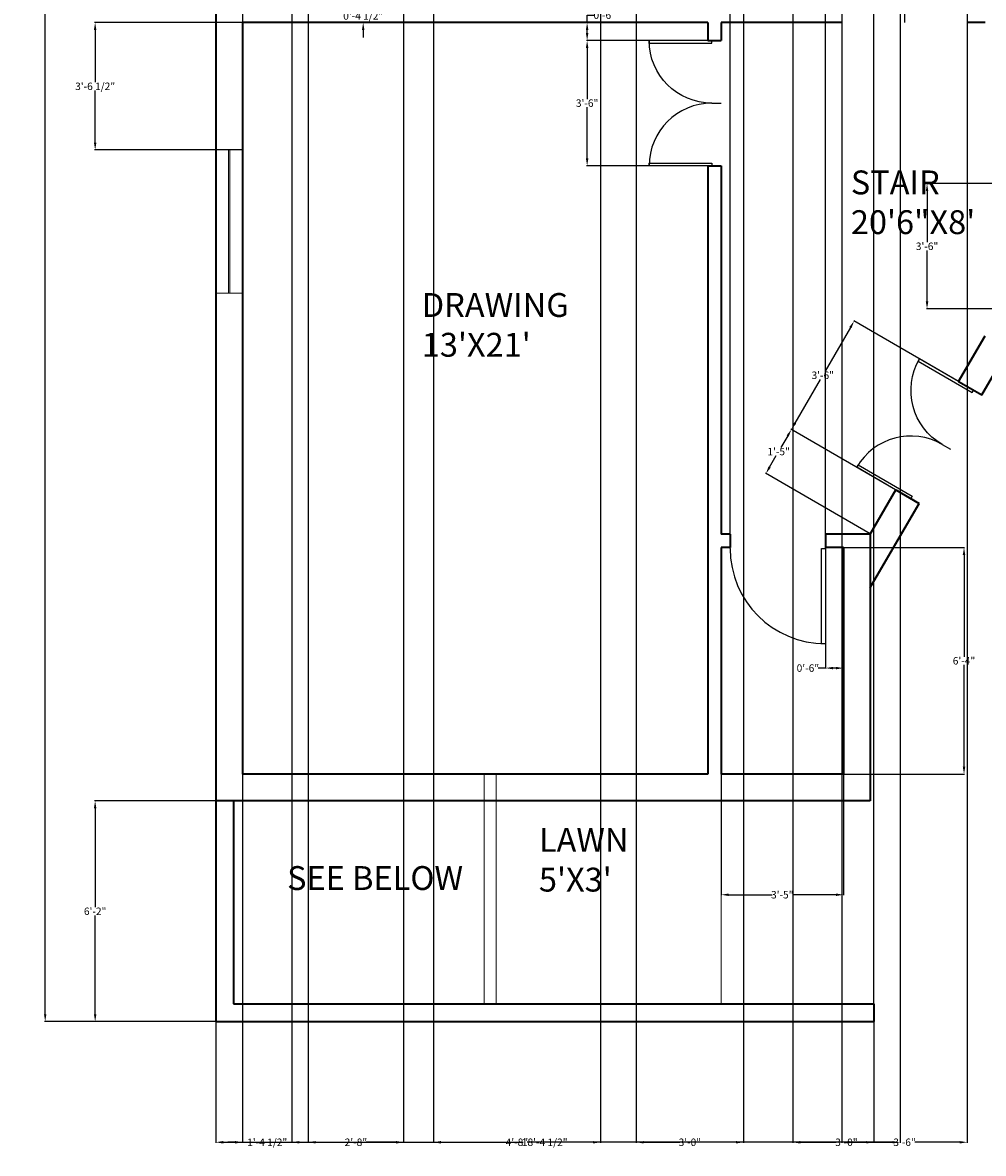
# Model space of a CAD drawing. Units: inches. Extents: x 1737 to 2270, y 2551 to 3419.
# Tile 1 of 4: x 1737 to 2060, y 2551 to 2930. Entities that reach past the tile are written whole.
import ezdxf

# ---------------------------------------------------------------- set-up
doc = ezdxf.new("R2010")
doc.units = ezdxf.units.IN
doc.header["$MEASUREMENT"] = 0
doc.layers.get('0').update_dxf_attribs({"color": 60})
for name, color, linetype, lineweight in [('A-ANNO-DIMS', 2, 'Continuous', 18), ('A-ANNO-TEXT', 231, 'Continuous', 18), ('A-AREA-IDEN', 231, 'Continuous', 18), ('DOOR', 20, 'Continuous', 25), ('L-SITE', 3, 'Continuous', 18), ('WALL', 60, 'Continuous', 35), ('WINDOW', 30, 'Continuous', 18)]:
    doc.layers.add(name, color=color, linetype=linetype, lineweight=lineweight)
doc.styles.get("Standard").update_dxf_attribs({"font": 'arial.ttf'})
doc.dimstyles.get("Standard").update_dxf_attribs({"dimtxt": 2.5, "dimasz": 2.5, "dimexe": 0.18, "dimexo": 0.0625, "dimgap": 0.09, "dimtad": 0, "dimtih": 1, "dimtoh": 1, "dimzin": 0, "dimdsep": 46, "dimlunit": 3, "dimtxsty": 'Standard', "dimcen": 0.09, "dimadec": 0, "dimazin": 0, "dimtfac": 1, "dimtofl": 0, "dimtmove": 0, "dimatfit": 3, "dimfxl": 1, "dimtolj": 1, "dimtzin": 0, "dimarcsym": 0})

# ---------------------------------------------------------------- blocks, each defined once
blk = doc.blocks.new('*U2')
for p, q in [((0, 0), (0, -6)), ((40, 0), (40, -6))]:
    blk.add_line(p, q)
blk.add_lwpolyline([(0, 0), (0, 40), (1.75, 40), (1.75, 0)], close=True)
blk.add_arc((0, 0), 40, 0, 90)
blk = doc.blocks.new('*D5')
at = {"layer": 'A-ANNO-DIMS', "color": 0, "lineweight": -2, "transparency": 16777216}
for p, q in [((1802.15, 3375.16), (1744.83, 3375.16)), ((1745.01, 3372.66), (1745.01, 2989.33)), ((1745.01, 2597.66), (1745.01, 2980.98)), ((1802.15, 2595.16), (1744.83, 2595.16))]:
    blk.add_line(p, q, dxfattribs=at)
at = {"layer": 'A-ANNO-DIMS', "color": 0, "transparency": 16777216}
for points in [[(1744.59, 3372.66), (1745.42, 3372.66), (1745.01, 3375.16)], [(1744.59, 2597.66), (1745.42, 2597.66), (1745.01, 2595.16)]]:
    blk.add_solid(points, dxfattribs=at)
at = {"layer": 'Defpoints', "color": 0, "transparency": 16777216}
for p in [(1802.21, 3375.16), (1745.01, 2595.16), (1802.21, 2595.16)]:
    blk.add_point(p, dxfattribs=at)
at = {"layer": 'A-ANNO-DIMS', "color": 0, "transparency": 16777216, "insert": (1745.01, 2985.16), "char_height": 8, "attachment_point": 5}
blk.add_mtext("\\A1;65'", dxfattribs=at)
blk = doc.blocks.new('WIN-48IN')
for p, q in [((4.25, 48), (4.25, 0)), ((4.75, 48), (4.75, 0))]:
    blk.add_line(p, q)
blk.add_lwpolyline([(0, 48), (0, 0), (9, 0), (9, 48)], close=True)
blk = doc.blocks.new('*D13')
at = {"layer": 'A-ANNO-DIMS', "color": 0, "lineweight": -2, "transparency": 16777216}
for p, q in [((1811.15, 2930.16), (1761.58, 2930.16)), ((1761.76, 2927.66), (1761.76, 2910.19)), ((1761.76, 2889.95), (1761.76, 2907.42)), ((1811.15, 2887.45), (1761.58, 2887.45))]:
    blk.add_line(p, q, dxfattribs=at)
at = {"layer": 'A-ANNO-DIMS', "color": 0, "transparency": 16777216}
for points in [[(1761.34, 2927.66), (1762.18, 2927.66), (1761.76, 2930.16)], [(1761.34, 2889.95), (1762.18, 2889.95), (1761.76, 2887.45)]]:
    blk.add_solid(points, dxfattribs=at)
at = {"layer": 'Defpoints', "color": 0, "transparency": 16777216}
for p in [(1811.21, 2930.16), (1761.76, 2887.45), (1811.21, 2887.45)]:
    blk.add_point(p, dxfattribs=at)
at = {"layer": 'A-ANNO-DIMS', "color": 0, "transparency": 16777216, "insert": (1761.76, 2908.8), "char_height": 2.5, "attachment_point": 5}
blk.add_mtext('\\A1;3\'-6 1/2"', dxfattribs=at)
blk = doc.blocks.new('*D18')
at = {"layer": 'A-ANNO-DIMS', "color": 0, "lineweight": -2, "transparency": 16777216}
for p, q in [((1811.21, 3366.1), (1811.21, 2554.53)), ((1827.73, 3366.1), (1827.73, 2554.53)), ((1808.71, 2554.71), (1806.21, 2554.71)), ((1830.23, 2554.71), (1832.73, 2554.71))]:
    blk.add_line(p, q, dxfattribs=at)
at = {"layer": 'A-ANNO-DIMS', "color": 0, "transparency": 16777216}
for points in [[(1808.71, 2555.12), (1808.71, 2554.29), (1811.21, 2554.71)], [(1830.23, 2555.12), (1830.23, 2554.29), (1827.73, 2554.71)]]:
    blk.add_solid(points, dxfattribs=at)
at = {"layer": 'Defpoints', "color": 0, "transparency": 16777216}
for p in [(1811.21, 3366.16), (1827.73, 3366.16), (1827.73, 2554.71)]:
    blk.add_point(p, dxfattribs=at)
at = {"layer": 'A-ANNO-DIMS', "color": 0, "transparency": 16777216, "insert": (1819.47, 2554.71), "char_height": 2.5, "attachment_point": 5}
blk.add_mtext('\\A1;1\'-4 1/2"', dxfattribs=at)
blk = doc.blocks.new('*D20')
at = {"layer": 'A-ANNO-DIMS', "color": 0, "lineweight": -2, "transparency": 16777216}
for p, q in [((2022.87, 2595.22), (2022.87, 3415.79)), ((2025.37, 3415.61), (2107.86, 3415.61)), ((2204.71, 3415.61), (2122.22, 3415.61)), ((2207.21, 2595.22), (2207.21, 3415.79))]:
    blk.add_line(p, q, dxfattribs=at)
at = {"layer": 'A-ANNO-DIMS', "color": 0, "transparency": 16777216}
for points in [[(2025.37, 3416.02), (2025.37, 3415.19), (2022.87, 3415.61)], [(2204.71, 3416.02), (2204.71, 3415.19), (2207.21, 3415.61)]]:
    blk.add_solid(points, dxfattribs=at)
at = {"layer": 'Defpoints', "color": 0, "transparency": 16777216}
for p in [(2207.21, 3415.61), (2022.87, 2595.16), (2207.21, 2595.16)]:
    blk.add_point(p, dxfattribs=at)
at = {"layer": 'A-ANNO-DIMS', "color": 0, "transparency": 16777216, "insert": (2115.04, 3415.61), "char_height": 2.5, "attachment_point": 5}
blk.add_mtext('\\A1;15\'-4 1/2"', dxfattribs=at)
blk = doc.blocks.new('*D21')
at = {"layer": 'A-ANNO-DIMS', "color": 0, "lineweight": -2, "transparency": 16777216}
for p, q in [((1802.21, 2595.1), (1802.21, 2554.53)), ((2022.87, 2595.1), (2022.87, 2554.53)), ((1804.71, 2554.71), (1905.36, 2554.71)), ((2020.37, 2554.71), (1919.72, 2554.71))]:
    blk.add_line(p, q, dxfattribs=at)
at = {"layer": 'A-ANNO-DIMS', "color": 0, "transparency": 16777216}
for points in [[(1804.71, 2555.12), (1804.71, 2554.29), (1802.21, 2554.71)], [(2020.37, 2555.12), (2020.37, 2554.29), (2022.87, 2554.71)]]:
    blk.add_solid(points, dxfattribs=at)
at = {"layer": 'Defpoints', "color": 0, "transparency": 16777216}
for p in [(1802.21, 2595.16), (2022.87, 2595.16), (2022.87, 2554.71)]:
    blk.add_point(p, dxfattribs=at)
at = {"layer": 'A-ANNO-DIMS', "color": 0, "transparency": 16777216, "insert": (1912.54, 2554.71), "char_height": 2.5, "attachment_point": 5}
blk.add_mtext('\\A1;18\'-4 1/2"', dxfattribs=at)
blk = doc.blocks.new('*D22')
at = {"layer": 'A-ANNO-DIMS', "color": 0, "lineweight": -2, "transparency": 16777216}
for p, q in [((1802.15, 2669.16), (1761.58, 2669.16)), ((1761.76, 2666.66), (1761.76, 2633.52)), ((1761.76, 2597.66), (1761.76, 2630.79)), ((1802.15, 2595.16), (1761.58, 2595.16))]:
    blk.add_line(p, q, dxfattribs=at)
at = {"layer": 'A-ANNO-DIMS', "color": 0, "transparency": 16777216}
for points in [[(1761.34, 2666.66), (1762.18, 2666.66), (1761.76, 2669.16)], [(1761.34, 2597.66), (1762.18, 2597.66), (1761.76, 2595.16)]]:
    blk.add_solid(points, dxfattribs=at)
at = {"layer": 'Defpoints', "color": 0, "transparency": 16777216}
for p in [(1761.76, 2669.16), (1802.21, 2669.16), (1802.21, 2595.16)]:
    blk.add_point(p, dxfattribs=at)
at = {"layer": 'A-ANNO-DIMS', "color": 0, "transparency": 16777216, "insert": (1761.76, 2632.16), "char_height": 2.5, "attachment_point": 5}
blk.add_mtext('\\A1;6\'-2"', dxfattribs=at)
blk = doc.blocks.new('*D23')
at = {"layer": 'A-ANNO-DIMS', "color": 0, "lineweight": -2, "transparency": 16777216}
for p, q in [((1943.21, 3123.6), (1943.21, 2554.53)), ((1979.21, 3123.6), (1979.21, 2554.53)), ((1945.71, 2554.71), (1957.8, 2554.71)), ((1976.71, 2554.71), (1964.62, 2554.71))]:
    blk.add_line(p, q, dxfattribs=at)
at = {"layer": 'A-ANNO-DIMS', "color": 0, "transparency": 16777216}
for points in [[(1945.71, 2555.12), (1945.71, 2554.29), (1943.21, 2554.71)], [(1976.71, 2555.12), (1976.71, 2554.29), (1979.21, 2554.71)]]:
    blk.add_solid(points, dxfattribs=at)
at = {"layer": 'Defpoints', "color": 0, "transparency": 16777216}
for p in [(1943.21, 3123.66), (1979.21, 3123.66), (1979.21, 2554.71)]:
    blk.add_point(p, dxfattribs=at)
at = {"layer": 'A-ANNO-DIMS', "color": 0, "transparency": 16777216, "insert": (1961.21, 2554.71), "char_height": 2.5, "attachment_point": 5}
blk.add_mtext('\\A1;3\'-0"', dxfattribs=at)
blk = doc.blocks.new('*D24')
at = {"layer": 'A-ANNO-DIMS', "color": 0, "lineweight": -2, "transparency": 16777216}
for p, q in [((1833.21, 3284.1), (1833.21, 2554.53)), ((1865.21, 3284.1), (1865.21, 2554.53)), ((1835.71, 2554.71), (1845.77, 2554.71)), ((1862.71, 2554.71), (1852.64, 2554.71))]:
    blk.add_line(p, q, dxfattribs=at)
at = {"layer": 'A-ANNO-DIMS', "color": 0, "transparency": 16777216}
for points in [[(1835.71, 2555.12), (1835.71, 2554.29), (1833.21, 2554.71)], [(1862.71, 2555.12), (1862.71, 2554.29), (1865.21, 2554.71)]]:
    blk.add_solid(points, dxfattribs=at)
at = {"layer": 'Defpoints', "color": 0, "transparency": 16777216}
for p in [(1833.21, 3284.16), (1865.21, 3284.16), (1865.21, 2554.71)]:
    blk.add_point(p, dxfattribs=at)
at = {"layer": 'A-ANNO-DIMS', "color": 0, "transparency": 16777216, "insert": (1849.21, 2554.71), "char_height": 2.5, "attachment_point": 5}
blk.add_mtext('\\A1;2\'-8"', dxfattribs=at)
blk = doc.blocks.new('*D25')
at = {"layer": 'A-ANNO-DIMS', "color": 0, "lineweight": -2, "transparency": 16777216}
for p, q in [((2012.21, 2930.1), (2012.21, 2554.53)), ((2054.21, 2930.1), (2054.21, 2554.53)), ((2014.71, 2554.71), (2029.8, 2554.71)), ((2051.71, 2554.71), (2036.62, 2554.71))]:
    blk.add_line(p, q, dxfattribs=at)
at = {"layer": 'A-ANNO-DIMS', "color": 0, "transparency": 16777216}
for points in [[(2014.71, 2555.12), (2014.71, 2554.29), (2012.21, 2554.71)], [(2051.71, 2555.12), (2051.71, 2554.29), (2054.21, 2554.71)]]:
    blk.add_solid(points, dxfattribs=at)
at = {"layer": 'Defpoints', "color": 0, "transparency": 16777216}
for p in [(2012.21, 2930.16), (2054.21, 2930.16), (2054.21, 2554.71)]:
    blk.add_point(p, dxfattribs=at)
at = {"layer": 'A-ANNO-DIMS', "color": 0, "transparency": 16777216, "insert": (2033.21, 2554.71), "char_height": 2.5, "attachment_point": 5}
blk.add_mtext('\\A1;3\'-6"', dxfattribs=at)
blk = doc.blocks.new('*D27')
at = {"layer": 'A-ANNO-DIMS', "color": 0, "lineweight": -2, "transparency": 16777216}
for p, q in [((1967.15, 2924.16), (1926.58, 2924.16)), ((1926.76, 2921.66), (1926.76, 2904.53)), ((1926.76, 2884.66), (1926.76, 2901.79)), ((1967.15, 2882.16), (1926.58, 2882.16))]:
    blk.add_line(p, q, dxfattribs=at)
at = {"layer": 'A-ANNO-DIMS', "color": 0, "transparency": 16777216}
for points in [[(1926.34, 2921.66), (1927.18, 2921.66), (1926.76, 2924.16)], [(1926.34, 2884.66), (1927.18, 2884.66), (1926.76, 2882.16)]]:
    blk.add_solid(points, dxfattribs=at)
at = {"layer": 'Defpoints', "color": 0, "transparency": 16777216}
for p in [(1926.76, 2924.16), (1967.21, 2924.16), (1967.21, 2882.16)]:
    blk.add_point(p, dxfattribs=at)
at = {"layer": 'A-ANNO-DIMS', "color": 0, "transparency": 16777216, "insert": (1926.76, 2903.16), "char_height": 2.5, "attachment_point": 5}
blk.add_mtext('\\A1;3\'-6"', dxfattribs=at)
blk = doc.blocks.new('*D28')
at = {"layer": 'A-ANNO-DIMS', "color": 0, "lineweight": -2, "transparency": 16777216}
for p, q in [((2051.26, 2809.83), (2016.16, 2830.16)), ((2015.06, 2827.91), (2006.58, 2813.26)), ((1996.52, 2795.89), (2005, 2810.53)), ((2030.22, 2773.49), (1995.11, 2793.81))]:
    blk.add_line(p, q, dxfattribs=at)
at = {"layer": 'A-ANNO-DIMS', "color": 0, "transparency": 16777216}
for points in [[(2014.7, 2828.11), (2015.42, 2827.7), (2016.31, 2830.07)], [(1996.16, 2796.09), (1996.88, 2795.68), (1995.27, 2793.72)]]:
    blk.add_solid(points, dxfattribs=at)
at = {"layer": 'Defpoints', "color": 0, "transparency": 16777216}
for p in [(2016.31, 2830.07), (2051.32, 2809.8), (2030.28, 2773.45)]:
    blk.add_point(p, dxfattribs=at)
at = {"layer": 'A-ANNO-DIMS', "color": 0, "transparency": 16777216, "insert": (2005.79, 2811.9), "char_height": 2.5, "attachment_point": 5}
blk.add_mtext('\\A1;3\'-6"', dxfattribs=at)
blk = doc.blocks.new('*D29')
at = {"layer": 'A-ANNO-DIMS', "color": 0, "lineweight": -2, "transparency": 16777216}
for p, q in [((1974.71, 2758.72), (1974.71, 3415.79)), ((1977.21, 3415.61), (1987.27, 3415.61)), ((2004.21, 3415.61), (1994.14, 3415.61)), ((2006.71, 2758.72), (2006.71, 3415.79))]:
    blk.add_line(p, q, dxfattribs=at)
at = {"layer": 'A-ANNO-DIMS', "color": 0, "transparency": 16777216}
for points in [[(1977.21, 3416.02), (1977.21, 3415.19), (1974.71, 3415.61)], [(2004.21, 3416.02), (2004.21, 3415.19), (2006.71, 3415.61)]]:
    blk.add_solid(points, dxfattribs=at)
at = {"layer": 'Defpoints', "color": 0, "transparency": 16777216}
for p in [(2006.71, 3415.61), (1974.71, 2758.66), (2006.71, 2758.66)]:
    blk.add_point(p, dxfattribs=at)
at = {"layer": 'A-ANNO-DIMS', "color": 0, "transparency": 16777216, "insert": (1990.71, 3415.61), "char_height": 2.5, "attachment_point": 5}
blk.add_mtext('\\A1;2\'-8"', dxfattribs=at)
blk = doc.blocks.new('*D30')
at = {"layer": 'A-ANNO-DIMS', "color": 0, "lineweight": -2, "transparency": 16777216}
for p, q in [((2081.15, 2876.16), (2040.58, 2876.16)), ((2040.76, 2873.66), (2040.76, 2856.53)), ((2040.76, 2836.66), (2040.76, 2853.79)), ((2081.15, 2834.16), (2040.58, 2834.16))]:
    blk.add_line(p, q, dxfattribs=at)
at = {"layer": 'A-ANNO-DIMS', "color": 0, "transparency": 16777216}
for points in [[(2040.34, 2873.66), (2041.18, 2873.66), (2040.76, 2876.16)], [(2040.34, 2836.66), (2041.18, 2836.66), (2040.76, 2834.16)]]:
    blk.add_solid(points, dxfattribs=at)
at = {"layer": 'Defpoints', "color": 0, "transparency": 16777216}
for p in [(2040.76, 2876.16), (2081.21, 2876.16), (2081.21, 2834.16)]:
    blk.add_point(p, dxfattribs=at)
at = {"layer": 'A-ANNO-DIMS', "color": 0, "transparency": 16777216, "insert": (2040.76, 2855.16), "char_height": 2.5, "attachment_point": 5}
blk.add_mtext('\\A1;3\'-6"', dxfattribs=at)
blk = doc.blocks.new('*D34')
at = {"layer": 'A-ANNO-DIMS', "color": 0, "lineweight": -2, "transparency": 16777216}
for p, q in [((1995.71, 3123.6), (1995.71, 2554.53)), ((2031.71, 3123.6), (2031.71, 2554.53)), ((1998.21, 2554.71), (2010.3, 2554.71)), ((2029.21, 2554.71), (2017.12, 2554.71))]:
    blk.add_line(p, q, dxfattribs=at)
at = {"layer": 'A-ANNO-DIMS', "color": 0, "transparency": 16777216}
for points in [[(1998.21, 2555.12), (1998.21, 2554.29), (1995.71, 2554.71)], [(2029.21, 2555.12), (2029.21, 2554.29), (2031.71, 2554.71)]]:
    blk.add_solid(points, dxfattribs=at)
at = {"layer": 'Defpoints', "color": 0, "transparency": 16777216}
for p in [(1995.71, 3123.66), (2031.71, 3123.66), (2031.71, 2554.71)]:
    blk.add_point(p, dxfattribs=at)
at = {"layer": 'A-ANNO-DIMS', "color": 0, "transparency": 16777216, "insert": (2013.71, 2554.71), "char_height": 2.5, "attachment_point": 5}
blk.add_mtext('\\A1;3\'-0"', dxfattribs=at)
blk = doc.blocks.new('*D39')
at = {"layer": 'A-ANNO-DIMS', "color": 0, "lineweight": -2, "transparency": 16777216}
for p, q in [((1875.21, 3366.1), (1875.21, 2554.53)), ((1931.21, 3366.1), (1931.21, 2554.53)), ((1877.71, 2554.71), (1899.75, 2554.71)), ((1928.71, 2554.71), (1906.67, 2554.71))]:
    blk.add_line(p, q, dxfattribs=at)
at = {"layer": 'A-ANNO-DIMS', "color": 0, "transparency": 16777216}
for points in [[(1877.71, 2555.12), (1877.71, 2554.29), (1875.21, 2554.71)], [(1928.71, 2555.12), (1928.71, 2554.29), (1931.21, 2554.71)]]:
    blk.add_solid(points, dxfattribs=at)
at = {"layer": 'Defpoints', "color": 0, "transparency": 16777216}
for p in [(1875.21, 3366.16), (1931.21, 3366.16), (1931.21, 2554.71)]:
    blk.add_point(p, dxfattribs=at)
at = {"layer": 'A-ANNO-DIMS', "color": 0, "transparency": 16777216, "insert": (1903.21, 2554.71), "char_height": 2.5, "attachment_point": 5}
blk.add_mtext('\\A1;4\'-8"', dxfattribs=at)
blk = doc.blocks.new('*D44')
at = {"layer": 'A-ANNO-DIMS', "color": 0, "lineweight": -2, "transparency": 16777216}
for p, q in [((1971.71, 2678.1), (1971.71, 2637.53)), ((2012.71, 2678.1), (2012.71, 2637.53)), ((1974.21, 2637.71), (1988.8, 2637.71)), ((2010.21, 2637.71), (1995.62, 2637.71))]:
    blk.add_line(p, q, dxfattribs=at)
at = {"layer": 'A-ANNO-DIMS', "color": 0, "transparency": 16777216}
for points in [[(1974.21, 2638.12), (1974.21, 2637.29), (1971.71, 2637.71)], [(2010.21, 2638.12), (2010.21, 2637.29), (2012.71, 2637.71)]]:
    blk.add_solid(points, dxfattribs=at)
at = {"layer": 'Defpoints', "color": 0, "transparency": 16777216}
for p in [(1971.71, 2678.16), (2012.71, 2678.16), (1971.71, 2637.71)]:
    blk.add_point(p, dxfattribs=at)
at = {"layer": 'A-ANNO-DIMS', "color": 0, "transparency": 16777216, "insert": (1992.21, 2637.71), "char_height": 2.5, "attachment_point": 5}
blk.add_mtext('\\A1;3\'-5"', dxfattribs=at)
blk = doc.blocks.new('*D45')
at = {"layer": 'A-ANNO-DIMS', "color": 0, "lineweight": -2, "transparency": 16777216}
for p, q in [((2012.77, 2754.16), (2053.34, 2754.16)), ((2053.16, 2751.66), (2053.16, 2717.52)), ((2053.16, 2680.66), (2053.16, 2714.79)), ((2012.77, 2678.16), (2053.34, 2678.16))]:
    blk.add_line(p, q, dxfattribs=at)
at = {"layer": 'A-ANNO-DIMS', "color": 0, "transparency": 16777216}
for points in [[(2052.74, 2751.66), (2053.58, 2751.66), (2053.16, 2754.16)], [(2052.74, 2680.66), (2053.58, 2680.66), (2053.16, 2678.16)]]:
    blk.add_solid(points, dxfattribs=at)
at = {"layer": 'Defpoints', "color": 0, "transparency": 16777216}
for p in [(2012.71, 2754.16), (2012.71, 2678.16), (2053.16, 2678.16)]:
    blk.add_point(p, dxfattribs=at)
at = {"layer": 'A-ANNO-DIMS', "color": 0, "transparency": 16777216, "insert": (2053.16, 2716.16), "char_height": 2.5, "attachment_point": 5}
blk.add_mtext('\\A1;6\'-4"', dxfattribs=at)
blk = doc.blocks.new('*D47')
at = {"layer": 'A-ANNO-DIMS', "color": 0, "lineweight": -2, "transparency": 16777216}
for p, q in [((1926.76, 2930.16), (1926.76, 2932.66)), ((1926.76, 2932.66), (1929.26, 2932.66)), ((1967.15, 2930.16), (1926.58, 2930.16)), ((1926.76, 2926.66), (1926.76, 2927.66)), ((1967.15, 2924.16), (1926.58, 2924.16))]:
    blk.add_line(p, q, dxfattribs=at)
at = {"layer": 'A-ANNO-DIMS', "color": 0, "transparency": 16777216}
for points in [[(1926.34, 2927.66), (1927.18, 2927.66), (1926.76, 2930.16)], [(1926.34, 2926.66), (1927.18, 2926.66), (1926.76, 2924.16)]]:
    blk.add_solid(points, dxfattribs=at)
at = {"layer": 'Defpoints', "color": 0, "transparency": 16777216}
for p in [(1926.76, 2930.16), (1967.21, 2930.16), (1967.21, 2924.16)]:
    blk.add_point(p, dxfattribs=at)
at = {"layer": 'A-ANNO-DIMS', "color": 0, "transparency": 16777216, "insert": (1932.67, 2932.66), "char_height": 2.5, "attachment_point": 5}
blk.add_mtext('\\A1;0\'-6"', dxfattribs=at)
blk = doc.blocks.new('*D49')
at = {"layer": 'A-ANNO-DIMS', "color": 0, "lineweight": -2, "transparency": 16777216}
for p, q in [((1994.02, 2791.56), (1991.78, 2787.69)), ((2030.22, 2773.49), (1995.11, 2793.81)), ((1987.95, 2781.09), (1990.19, 2784.96)), ((2021.65, 2758.69), (1986.55, 2779.02))]:
    blk.add_line(p, q, dxfattribs=at)
at = {"layer": 'A-ANNO-DIMS', "color": 0, "transparency": 16777216}
for points in [[(1993.66, 2791.77), (1994.38, 2791.35), (1995.27, 2793.72)], [(1987.59, 2781.3), (1988.32, 2780.88), (1986.7, 2778.92)]]:
    blk.add_solid(points, dxfattribs=at)
at = {"layer": 'Defpoints', "color": 0, "transparency": 16777216}
for p in [(1995.27, 2793.72), (2030.28, 2773.45), (2021.71, 2758.66)]:
    blk.add_point(p, dxfattribs=at)
at = {"layer": 'A-ANNO-DIMS', "color": 0, "transparency": 16777216, "insert": (1990.99, 2786.32), "char_height": 2.5, "attachment_point": 5}
blk.add_mtext('\\A1;1\'-5"', dxfattribs=at)
blk = doc.blocks.new('*D50')
at = {"layer": 'A-ANNO-DIMS', "color": 0, "lineweight": -2, "transparency": 16777216}
for p, q in [((2006.71, 2754.1), (2006.71, 2713.53)), ((2012.71, 2754.1), (2012.71, 2713.53)), ((2006.71, 2713.71), (2004.21, 2713.71)), ((2010.21, 2713.71), (2009.21, 2713.71))]:
    blk.add_line(p, q, dxfattribs=at)
at = {"layer": 'A-ANNO-DIMS', "color": 0, "transparency": 16777216}
for points in [[(2009.21, 2714.12), (2009.21, 2713.29), (2006.71, 2713.71)], [(2010.21, 2714.12), (2010.21, 2713.29), (2012.71, 2713.71)]]:
    blk.add_solid(points, dxfattribs=at)
at = {"layer": 'Defpoints', "color": 0, "transparency": 16777216}
for p in [(2006.71, 2754.16), (2012.71, 2754.16), (2006.71, 2713.71)]:
    blk.add_point(p, dxfattribs=at)
at = {"layer": 'A-ANNO-DIMS', "color": 0, "transparency": 16777216, "insert": (2000.8, 2713.71), "char_height": 2.5, "attachment_point": 5}
blk.add_mtext('\\A1;0\'-6"', dxfattribs=at)
blk = doc.blocks.new('*D51')
at = {"layer": 'A-ANNO-DIMS', "color": 0, "lineweight": -2, "transparency": 16777216}
for p, q in [((1851.66, 2937.16), (1851.66, 2939.66)), ((1811.27, 2934.66), (1851.84, 2934.66)), ((1811.27, 2930.16), (1851.84, 2930.16)), ((1851.66, 2927.66), (1851.66, 2925.16))]:
    blk.add_line(p, q, dxfattribs=at)
at = {"layer": 'A-ANNO-DIMS', "color": 0, "transparency": 16777216}
for points in [[(1851.24, 2937.16), (1852.08, 2937.16), (1851.66, 2934.66)], [(1851.24, 2927.66), (1852.08, 2927.66), (1851.66, 2930.16)]]:
    blk.add_solid(points, dxfattribs=at)
at = {"layer": 'Defpoints', "color": 0, "transparency": 16777216}
for p in [(1811.21, 2934.66), (1811.21, 2930.16), (1851.66, 2930.16)]:
    blk.add_point(p, dxfattribs=at)
at = {"layer": 'A-ANNO-DIMS', "color": 0, "transparency": 16777216, "insert": (1851.66, 2932.41), "char_height": 2.5, "attachment_point": 5}
blk.add_mtext('\\A1;0\'-4 1/2"', dxfattribs=at)

msp = doc.modelspace()

# ---------------------------------------------------------------- linework, layer by layer
at = {"layer": 'L-SITE'}
for p, q in [((1892.209, 2678.158), (1892.209, 2601.158)), ((1896.209, 2678.158), (1896.209, 2601.158)), ((1971.709, 2669.158), (1971.709, 2601.158))]:
    msp.add_line(p, q, dxfattribs=at)
at = {"layer": 'WALL'}
for p, q in [((1802.209, 3375.158), (1802.209, 2669.158)), ((1811.209, 2930.158), (1811.209, 2678.158)), ((1967.209, 2930.158), (1811.209, 2930.158)), ((1967.209, 2930.158), (1967.209, 2924.158)), ((1971.709, 2930.158), (1971.709, 2924.158)), ((2012.209, 2930.158), (1971.709, 2930.158)), ((2060.209, 2930.158), (2054.209, 2930.158)), ((1967.209, 2924.158), (1971.709, 2924.158)), ((1967.209, 2882.158), (1971.709, 2882.158)), ((1967.209, 2882.158), (1967.209, 2678.158)), ((1971.709, 2882.158), (1971.709, 2758.658)), ((2051.319, 2809.803), (2060.209, 2825.158)), ((2059.108, 2805.293), (2070.608, 2825.158)), ((2051.319, 2809.803), (2059.108, 2805.293)), ((2021.709, 2758.658), (2030.275, 2773.455)), ((2030.275, 2773.455), (2038.064, 2768.945)), ((2021.709, 2740.695), (2038.064, 2768.945)), ((1974.709, 2758.658), (1971.709, 2758.658)), ((1974.709, 2758.658), (1974.709, 2754.158)), ((2021.709, 2758.658), (2006.709, 2758.658)), ((2006.709, 2758.658), (2006.709, 2754.158)), ((2021.709, 2758.658), (2021.709, 2669.158)), ((1971.709, 2754.158), (1971.709, 2678.158)), ((1974.709, 2754.158), (1971.709, 2754.158)), ((2012.709, 2754.158), (2006.709, 2754.158)), ((2012.709, 2754.158), (2012.709, 2678.158)), ((1967.209, 2678.158), (1811.209, 2678.158)), ((2012.709, 2678.158), (1971.709, 2678.158)), ((2021.709, 2669.158), (1802.209, 2669.158)), ((1802.209, 2669.158), (1802.209, 2595.158)), ((1808.209, 2669.158), (1808.209, 2601.158)), ((1808.209, 2601.158), (2022.872, 2601.158)), ((2022.872, 2601.158), (2022.872, 2595.158)), ((1802.209, 2595.158), (2022.872, 2595.158))]:
    msp.add_line(p, q, dxfattribs=at)

# ---------------------------------------------------------------- block references
at = {"layer": 'DOOR', "yscale": 0.5249999999999972, "zscale": 0.5249999999999972}
for p, xscale in [((2012.209, 2933.308), 0.5249999999999972), ((2054.209, 2933.308), -0.5249999999999972)]:
    msp.add_blockref('*U2', p, dxfattribs=dict(at, xscale=xscale))
at = {"layer": 'DOOR'}
for p, xscale, yscale, zscale, rotation in [((1968.559, 2924.158), -0.525, 0.525, 0.525, 90), ((1968.559, 2882.158), 0.525, 0.525, 0.525, 90), ((2056.382, 2806.872), -0.525, 0.525, 0.525, 59.93141717813752), ((2035.338, 2770.524), 0.525, 0.525, 0.525, 59.93141717813748), ((2006.709, 2753.858), 0.8, 0.8, 0.8, 180)]:
    msp.add_blockref('*U2', p, dxfattribs=dict(at, xscale=xscale, yscale=yscale, zscale=zscale, rotation=rotation))
at = {"layer": 'WINDOW'}
msp.add_blockref('WIN-48IN', (1802.209, 2839.449), dxfattribs=at)

# ---------------------------------------------------------------- texts
at = {"layer": 'A-ANNO-TEXT', "insert": (1826.137, 2647.307), "char_height": 8, "attachment_point": 1}
msp.add_mtext_dynamic_manual_height_columns('SEE BELOW', width=60.91246, gutter_width=1, heights=[0], dxfattribs=at)
at = {"layer": 'A-AREA-IDEN', "char_height": 8, "attachment_point": 1}
for s, insert in [('STAIR\\P20\'6"X8\'', (2015.204, 2880.576)), ("DRAWING\\P13'X21'", (1871.313, 2839.463)), ("LAWN\\P5'X3'", (1910.595, 2660.108))]:
    msp.add_mtext_dynamic_manual_height_columns(s, width=60.91246, gutter_width=1, heights=[0], dxfattribs=dict(at, insert=insert))

# ---------------------------------------------------------------- dimensions: what is measured, and where the dimension line sits
at = {"layer": 'A-ANNO-DIMS'}
for base, p1, p2, picture, middle in [((2006.709, 3415.608), (1974.709, 2758.658), (2006.709, 2758.658), '*D29', (1990.709, 3415.608)), ((2207.209, 3415.608), (2022.872, 2595.158), (2207.209, 2595.158), '*D20', (2115.041, 3415.608)), ((1827.725, 2554.708), (1811.209, 3366.158), (1827.725, 3366.158), '*D18', (1819.467, 2554.708)), ((1931.209, 2554.708), (1875.209, 3366.158), (1931.209, 3366.158), '*D39', (1903.209, 2554.708)), ((1865.209, 2554.708), (1833.209, 3284.158), (1865.209, 3284.158), '*D24', (1849.209, 2554.708)), ((1979.209, 2554.708), (1943.209, 3123.658), (1979.209, 3123.658), '*D23', (1961.209, 2554.708)), ((2031.709, 2554.708), (1995.709, 3123.658), (2031.709, 3123.658), '*D34', (2013.709, 2554.708)), ((2054.209, 2554.708), (2012.209, 2930.158), (2054.209, 2930.158), '*D25', (2033.209, 2554.708)), ((2022.872, 2554.708), (1802.209, 2595.158), (2022.872, 2595.158), '*D21', (1912.541, 2554.708))]:
    dim = msp.add_linear_dim(base=base, p1=p1, p2=p2, dimstyle='Standard', override={"dimdec": 1, "dimlfac": 1, "dimrnd": 0, "dimzin": 1, "dimdsep": 46, "dimlunit": 4, "dimfrac": 2}, dxfattribs=at)
    dim.commit()
    dim.dimension.update_dxf_attribs({"geometry": picture, "text_midpoint": middle})
dim = msp.add_aligned_dim(p1=(1802.209, 3375.158), p2=(1802.209, 2595.158), distance=-57.201, dimstyle='Standard', override={"dimtxt": 8, "dimclrd": 0, "dimclre": 0, "dimclrt": 0}, dxfattribs=at)
dim.commit()
dim.dimension.update_dxf_attribs({"geometry": '*D5', "text_midpoint": (1745.008, 2985.158)})
for base, p1, p2, angle, picture, middle in [((1851.659, 2930.158), (1811.209, 2934.658), (1811.209, 2930.158), 270, '*D51', (1851.659, 2932.408)), ((1926.759, 2930.158), (1967.209, 2924.158), (1967.209, 2930.158), 90, '*D47', (1932.672, 2932.658)), ((1761.759, 2887.449), (1811.209, 2930.158), (1811.209, 2887.449), 90, '*D13', (1761.759, 2908.803)), ((1926.759, 2924.158), (1967.209, 2882.158), (1967.209, 2924.158), 90, '*D27', (1926.759, 2903.158)), ((2040.759, 2876.158), (2081.209, 2834.158), (2081.209, 2876.158), 90, '*D30', (2040.759, 2855.158)), ((2016.312, 2830.07), (2030.275, 2773.455), (2051.319, 2809.803), 59.93142, '*D28', (2005.791, 2811.896)), ((1995.269, 2793.722), (2021.709, 2758.658), (2030.275, 2773.455), 59.93142, '*D49', (1990.986, 2786.323)), ((2006.709, 2713.708), (2012.709, 2754.158), (2006.709, 2754.158), 180, '*D50', (2000.796, 2713.708)), ((2053.159, 2678.158), (2012.709, 2754.158), (2012.709, 2678.158), 270, '*D45', (2053.159, 2716.158)), ((1971.709, 2637.708), (2012.709, 2678.158), (1971.709, 2678.158), 180, '*D44', (1992.209, 2637.708)), ((1761.759, 2669.158), (1802.209, 2595.158), (1802.209, 2669.158), 90, '*D22', (1761.759, 2632.158))]:
    dim = msp.add_linear_dim(base=base, p1=p1, p2=p2, angle=angle, dimstyle='Standard', override={"dimdec": 1, "dimlfac": 1, "dimrnd": 0, "dimzin": 1, "dimdsep": 46, "dimlunit": 4, "dimfrac": 2}, dxfattribs=at)
    dim.commit()
    dim.dimension.update_dxf_attribs({"geometry": picture, "text_midpoint": middle})

doc.saveas('drawing.dxf')
